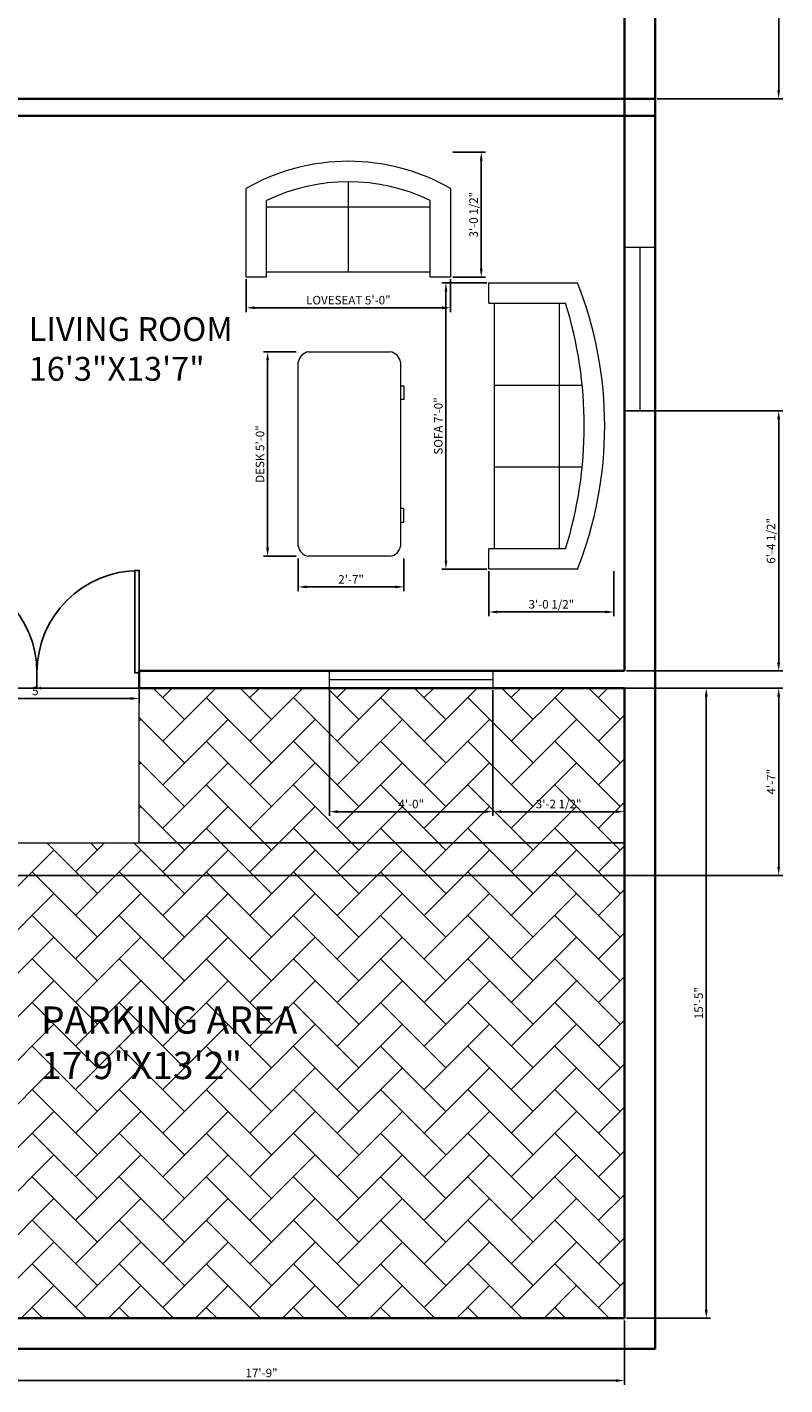
# Model space of a CAD drawing. Units: inches. Extents: x 3715 to 4224, y 2597 to 3354.
# Tile 3 of 5: x 4001 to 4224, y 2624 to 3023. Entities that reach past the tile are written whole.
import ezdxf

# ---------------------------------------------------------------- set-up
doc = ezdxf.new("R2010")
doc.units = ezdxf.units.IN
for name, color, linetype, lineweight in [('A-AREA-IDEN', 4, 'Continuous', 25), ('A-WALL', 7, 'Continuous', 35), ('DIM', 1, 'Continuous', 18), ('DOOR', 3, 'Continuous', 25), ('FURNITURES', 30, 'Continuous', 18), ('L-PAVE', 8, 'Continuous', 18), ('L-PAVE-PATT', 252, 'Continuous', 13), ('WINDOW', 6, 'Continuous', 20)]:
    doc.layers.add(name, color=color, linetype=linetype, lineweight=lineweight)
doc.styles.get("Standard").update_dxf_attribs({"font": 'arial.ttf'})
doc.dimstyles.new('ISO-25', dxfattribs={"dimtxt": 2.5, "dimasz": 2.5, "dimexe": 1.25, "dimexo": 0.625, "dimtad": 1, "dimlunit": 3, "dimtxsty": 'Standard', "dimcen": 2.5, "dimadec": 0, "dimazin": 0, "dimtfac": 1, "dimtmove": 0, "dimatfit": 3, "dimfxl": 1, "dimarcsym": 0})

# ---------------------------------------------------------------- blocks, each defined once
blk = doc.blocks.new('*U2')
for p, q in [((0, 0), (0, -6)), ((40, 0), (40, -6))]:
    blk.add_line(p, q)
blk.add_lwpolyline([(0, 0), (0, 40), (1.75, 40), (1.75, 0)], close=True)
blk.add_arc((0, 0), 40, 0, 90)
blk = doc.blocks.new('*U4')
for p, q in [((0, 0), (0, -6)), ((-40, 0), (-40, -6))]:
    blk.add_line(p, q)
blk.add_lwpolyline([(0, 0), (0, 40), (-1.75, 40), (-1.75, 0)], close=True)
blk.add_arc((0, 0), 40, 90, 180)
blk = doc.blocks.new('Desk - 30 x 60 in.')
for p, q in [((-26.999995, 0), (26.999995, 0)), ((-29.999995, -27), (-29.999995, -3)), ((29.999995, -3), (29.999995, -27)), ((26.999995, -30), (-26.999995, -30)), ((-20.000005, -30), (-20.000005, -31)), ((-20.000005, -31), (-16.000005, -31)), ((-16.000005, -31), (-16.000005, -30)), ((15.999995, -31), (15.999995, -30)), ((19.999995, -31), (15.999995, -31)), ((19.999995, -30), (19.999995, -31))]:
    blk.add_line(p, q)
for centre, start, end in [((-26.499995, -3.5), 98.1301, 171.8699), ((26.499995, -3.5), 8.130102, 81.8699), ((-26.499995, -26.5), 188.1301, 261.8699), ((26.499995, -26.5), 278.1301, 351.8699)]:
    blk.add_arc(centre, 3.535534, start, end)
blk = doc.blocks.new('Sofa - Roundback 7 ft.')
for p, q in [((-12.00002, -32.4421), (-12.00003, -6.5971)), ((11.99997, -32.4421), (11.99998, -6.5971)), ((-36.000027, -34), (-36.000027, -11.4696)), ((35.99998, -34), (35.99998, -11.4696)), ((-35.999844, -13.3819), (35.9998, -13.3819)), ((-36.000027, -32.4421), (35.99998, -32.4421))]:
    blk.add_line(p, q)
for points in [[(-36.000027, -34), (-42.000027, -34), (-42.000027, -8)], [(41.99998, -8), (41.99998, -34), (35.99998, -34)]]:
    blk.add_lwpolyline(points)
for centre, radius, start, end in [((0, -114.25), 114.25, 68.43141, 111.5686), ((-0.00001, -127.1968), 121.1968, 72.72033, 107.2797)]:
    blk.add_arc(centre, radius, start, end)
blk = doc.blocks.new('Sofa - Roundback Loveseat 5 ft.')
for p, q in [((0, -32.44198), (0, -5.99998)), ((-24, -33.99998), (-24, -11.46958)), ((24.00004, -33.99998), (24.00004, -11.46958)), ((-23.9998, -13.38178), (23.99986, -13.38178)), ((-24, -32.44198), (24.00004, -32.44198))]:
    blk.add_line(p, q)
for points in [[(-24, -33.99998), (-30, -33.99998), (-30, -7.99998)], [(30.00004, -7.99998), (30.00004, -33.99998), (24.00004, -33.99998)]]:
    blk.add_lwpolyline(points)
for centre, radius, start, end in [((0, -60.24998), 60.24998, 60.13715, 119.8628), ((0, -61.38438), 55.38444, 64.32083, 115.6792)]:
    blk.add_arc(centre, radius, start, end)
blk = doc.blocks.new('*D27')
at = {"layer": 'Defpoints', "color": 0, "transparency": 16777216}
for p in [(3963.48, 2643.93), (4176.48, 2643.93), (4176.48, 2625.63)]:
    blk.add_point(p, dxfattribs=at)
at = {"layer": 'DIM', "color": 0, "lineweight": -2, "transparency": 16777216}
for p, q in [((3963.48, 2643.31), (3963.48, 2624.38)), ((4176.48, 2643.31), (4176.48, 2624.38)), ((3965.98, 2625.63), (4173.98, 2625.63))]:
    blk.add_line(p, q, dxfattribs=at)
at = {"layer": 'DIM', "color": 0, "transparency": 16777216}
for points in [[(3965.98, 2626.04), (3965.98, 2625.21), (3963.48, 2625.63)], [(4173.98, 2626.04), (4173.98, 2625.21), (4176.48, 2625.63)]]:
    blk.add_solid(points, dxfattribs=at)
at = {"layer": 'DIM', "color": 0, "transparency": 16777216, "insert": (4069.98, 2627.53), "char_height": 2.5, "attachment_point": 5}
blk.add_mtext('17\'-9"', dxfattribs=at)
blk = doc.blocks.new('*D28')
at = {"layer": 'Defpoints', "color": 0, "transparency": 16777216}
for p in [(4176.48, 2828.93), (4176.48, 2643.93), (4200.53, 2643.93)]:
    blk.add_point(p, dxfattribs=at)
at = {"layer": 'DIM', "color": 0, "lineweight": -2, "transparency": 16777216}
for p, q in [((4177.1, 2828.93), (4201.78, 2828.93)), ((4200.53, 2826.43), (4200.53, 2646.43)), ((4177.1, 2643.93), (4201.78, 2643.93))]:
    blk.add_line(p, q, dxfattribs=at)
at = {"layer": 'DIM', "color": 0, "transparency": 16777216}
for points in [[(4200.11, 2826.43), (4200.95, 2826.43), (4200.53, 2828.93)], [(4200.11, 2646.43), (4200.95, 2646.43), (4200.53, 2643.93)]]:
    blk.add_solid(points, dxfattribs=at)
at = {"layer": 'DIM', "color": 0, "transparency": 16777216, "insert": (4198.63, 2736.43), "char_height": 2.5, "attachment_point": 5, "rotation": 90}
blk.add_mtext('15\'-5"', dxfattribs=at)
blk = doc.blocks.new('*D35')
at = {"layer": 'Defpoints', "color": 0, "transparency": 16777216}
for p in [(3974.06, 2828.93), (4034.06, 2828.93), (4034.06, 2825.86)]:
    blk.add_point(p, dxfattribs=at)
at = {"layer": 'DIM', "color": 0, "lineweight": -2, "transparency": 16777216}
for p, q in [((3974.06, 2828.31), (3974.06, 2824.61)), ((3976.56, 2825.86), (4031.56, 2825.86)), ((4034.06, 2828.31), (4034.06, 2824.61))]:
    blk.add_line(p, q, dxfattribs=at)
at = {"layer": 'DIM', "color": 0, "transparency": 16777216}
for points in [[(3976.56, 2826.28), (3976.56, 2825.45), (3974.06, 2825.86)], [(4031.56, 2826.28), (4031.56, 2825.45), (4034.06, 2825.86)]]:
    blk.add_solid(points, dxfattribs=at)
at = {"layer": 'DIM', "color": 0, "transparency": 16777216, "insert": (4004.06, 2827.76), "char_height": 2.5, "attachment_point": 5}
blk.add_mtext("5'", dxfattribs=at)
blk = doc.blocks.new('WIN-48IN-9IN-WALL')
blk.add_line((4.5, 48), (4.5, 0))
blk.add_lwpolyline([(0, 48), (9, 48), (9, 0), (0, 0)], close=True)
blk = doc.blocks.new('*D57')
at = {"layer": 'Defpoints', "color": 0, "transparency": 16777216}
for p in [(4071.76, 2927.61), (4080.76, 2927.61), (4080.76, 2867.61)]:
    blk.add_point(p, dxfattribs=at)
at = {"layer": 'DIM', "color": 0, "lineweight": -2, "transparency": 16777216}
for p, q in [((4080.14, 2927.61), (4070.51, 2927.61)), ((4071.76, 2870.11), (4071.76, 2925.11)), ((4080.14, 2867.61), (4070.51, 2867.61))]:
    blk.add_line(p, q, dxfattribs=at)
at = {"layer": 'DIM', "color": 0, "transparency": 16777216}
for points in [[(4071.35, 2925.11), (4072.18, 2925.11), (4071.76, 2927.61)], [(4071.35, 2870.11), (4072.18, 2870.11), (4071.76, 2867.61)]]:
    blk.add_solid(points, dxfattribs=at)
at = {"layer": 'DIM', "color": 0, "transparency": 16777216, "insert": (4069.85, 2897.61), "char_height": 2.5, "attachment_point": 5, "rotation": 90}
blk.add_mtext('DESK 5\'-0"', dxfattribs=at)
blk = doc.blocks.new('*D58')
at = {"layer": 'Defpoints', "color": 0, "transparency": 16777216}
for p in [(4080.76, 2867.61), (4111.76, 2867.61), (4080.76, 2858.61)]:
    blk.add_point(p, dxfattribs=at)
at = {"layer": 'DIM', "color": 0, "lineweight": -2, "transparency": 16777216}
for p, q in [((4080.76, 2866.98), (4080.76, 2857.36)), ((4111.76, 2866.98), (4111.76, 2857.36)), ((4109.26, 2858.61), (4083.26, 2858.61))]:
    blk.add_line(p, q, dxfattribs=at)
at = {"layer": 'DIM', "color": 0, "transparency": 16777216}
for points in [[(4083.26, 2859.02), (4083.26, 2858.19), (4080.76, 2858.61)], [(4109.26, 2859.02), (4109.26, 2858.19), (4111.76, 2858.61)]]:
    blk.add_solid(points, dxfattribs=at)
at = {"layer": 'DIM', "color": 0, "transparency": 16777216, "insert": (4096.26, 2860.49), "char_height": 2.5, "attachment_point": 5}
blk.add_mtext('2\'-7"', dxfattribs=at)
blk = doc.blocks.new('*D61')
at = {"layer": 'Defpoints', "color": 0, "transparency": 16777216}
for p in [(4136.71, 2947.86), (4124.11, 2863.86), (4136.71, 2863.86)]:
    blk.add_point(p, dxfattribs=at)
at = {"layer": 'DIM', "color": 0, "lineweight": -2, "transparency": 16777216}
for p, q in [((4136.09, 2947.86), (4122.86, 2947.86)), ((4124.11, 2945.36), (4124.11, 2866.36)), ((4136.09, 2863.86), (4122.86, 2863.86))]:
    blk.add_line(p, q, dxfattribs=at)
at = {"layer": 'DIM', "color": 0, "transparency": 16777216}
for points in [[(4123.7, 2945.36), (4124.53, 2945.36), (4124.11, 2947.86)], [(4123.7, 2866.36), (4124.53, 2866.36), (4124.11, 2863.86)]]:
    blk.add_solid(points, dxfattribs=at)
at = {"layer": 'DIM', "color": 0, "transparency": 16777216, "insert": (4122.19, 2905.86), "char_height": 2.5, "attachment_point": 5, "rotation": 90}
blk.add_mtext('SOFA 7\'-0"', dxfattribs=at)
blk = doc.blocks.new('*D62')
at = {"layer": 'Defpoints', "color": 0, "transparency": 16777216}
for p in [(4136.71, 2863.86), (4173.38, 2863.86), (4173.38, 2851.26)]:
    blk.add_point(p, dxfattribs=at)
at = {"layer": 'DIM', "color": 0, "lineweight": -2, "transparency": 16777216}
for p, q in [((4136.71, 2863.24), (4136.71, 2850.01)), ((4173.38, 2863.24), (4173.38, 2850.01)), ((4139.21, 2851.26), (4170.88, 2851.26))]:
    blk.add_line(p, q, dxfattribs=at)
at = {"layer": 'DIM', "color": 0, "transparency": 16777216}
for points in [[(4139.21, 2851.68), (4139.21, 2850.84), (4136.71, 2851.26)], [(4170.88, 2851.68), (4170.88, 2850.84), (4173.38, 2851.26)]]:
    blk.add_solid(points, dxfattribs=at)
at = {"layer": 'DIM', "color": 0, "transparency": 16777216, "insert": (4155.05, 2853.18), "char_height": 2.5, "attachment_point": 5}
blk.add_mtext('3\'-0 1/2"', dxfattribs=at)
blk = doc.blocks.new('*D63')
at = {"layer": 'Defpoints', "color": 0, "transparency": 16777216}
for p in [(4065.47, 2949.55), (4125.47, 2949.55), (4125.47, 2940.55)]:
    blk.add_point(p, dxfattribs=at)
at = {"layer": 'DIM', "color": 0, "lineweight": -2, "transparency": 16777216}
for p, q in [((4065.47, 2948.93), (4065.47, 2939.3)), ((4125.47, 2948.93), (4125.47, 2939.3)), ((4067.97, 2940.55), (4122.97, 2940.55))]:
    blk.add_line(p, q, dxfattribs=at)
at = {"layer": 'DIM', "color": 0, "transparency": 16777216}
for points in [[(4067.97, 2940.97), (4067.97, 2940.14), (4065.47, 2940.55)], [(4122.97, 2940.97), (4122.97, 2940.14), (4125.47, 2940.55)]]:
    blk.add_solid(points, dxfattribs=at)
at = {"layer": 'DIM', "color": 0, "transparency": 16777216, "insert": (4095.47, 2942.47), "char_height": 2.5, "attachment_point": 5}
blk.add_mtext('LOVESEAT 5\'-0"', dxfattribs=at)
blk = doc.blocks.new('*D64')
at = {"layer": 'Defpoints', "color": 0, "transparency": 16777216}
for p in [(4125.47, 2986.22), (4134.47, 2986.22), (4125.47, 2949.55)]:
    blk.add_point(p, dxfattribs=at)
at = {"layer": 'DIM', "color": 0, "lineweight": -2, "transparency": 16777216}
for p, q in [((4126.09, 2986.22), (4135.72, 2986.22)), ((4134.47, 2952.05), (4134.47, 2983.72)), ((4126.09, 2949.55), (4135.72, 2949.55))]:
    blk.add_line(p, q, dxfattribs=at)
at = {"layer": 'DIM', "color": 0, "transparency": 16777216}
for points in [[(4134.05, 2983.72), (4134.88, 2983.72), (4134.47, 2986.22)], [(4134.05, 2952.05), (4134.88, 2952.05), (4134.47, 2949.55)]]:
    blk.add_solid(points, dxfattribs=at)
at = {"layer": 'DIM', "color": 0, "transparency": 16777216, "insert": (4132.55, 2967.89), "char_height": 2.5, "attachment_point": 5, "rotation": 90}
blk.add_mtext('3\'-0 1/2"', dxfattribs=at)
blk = doc.blocks.new('*D82')
at = {"layer": 'Defpoints', "color": 0, "transparency": 16777216}
for p in [(3958.48, 2828.93), (4221.78, 2828.93), (3963.48, 2773.93)]:
    blk.add_point(p, dxfattribs=at)
at = {"layer": 'DIM', "color": 0, "lineweight": -2, "transparency": 16777216}
for p, q in [((3959.1, 2828.93), (4223.03, 2828.93)), ((4221.78, 2776.43), (4221.78, 2826.43)), ((3964.1, 2773.93), (4223.03, 2773.93))]:
    blk.add_line(p, q, dxfattribs=at)
at = {"layer": 'DIM', "color": 0, "transparency": 16777216}
for points in [[(4221.36, 2826.43), (4222.19, 2826.43), (4221.78, 2828.93)], [(4221.36, 2776.43), (4222.19, 2776.43), (4221.78, 2773.93)]]:
    blk.add_solid(points, dxfattribs=at)
at = {"layer": 'DIM', "color": 0, "transparency": 16777216, "insert": (4219.9, 2801.43), "char_height": 2.5, "attachment_point": 5, "rotation": 90}
blk.add_mtext('4\'-7"', dxfattribs=at)
blk = doc.blocks.new('*D86')
at = {"layer": 'Defpoints', "color": 0, "transparency": 16777216}
for p in [(4176.48, 2910.33), (4221.78, 2910.33), (4176.48, 2833.93)]:
    blk.add_point(p, dxfattribs=at)
at = {"layer": 'DIM', "color": 0, "lineweight": -2, "transparency": 16777216}
for p, q in [((4177.1, 2910.33), (4223.03, 2910.33)), ((4221.78, 2836.43), (4221.78, 2907.83)), ((4177.1, 2833.93), (4223.03, 2833.93))]:
    blk.add_line(p, q, dxfattribs=at)
at = {"layer": 'DIM', "color": 0, "transparency": 16777216}
for points in [[(4221.36, 2907.83), (4222.19, 2907.83), (4221.78, 2910.33)], [(4221.36, 2836.43), (4222.19, 2836.43), (4221.78, 2833.93)]]:
    blk.add_solid(points, dxfattribs=at)
at = {"layer": 'DIM', "color": 0, "transparency": 16777216, "insert": (4219.86, 2872.13), "char_height": 2.5, "attachment_point": 5, "rotation": 90}
blk.add_mtext('6\'-4 1/2"', dxfattribs=at)
blk = doc.blocks.new('*D87')
at = {"layer": 'Defpoints', "color": 0, "transparency": 16777216}
for p in [(4176.48, 3062.95), (4221.78, 3062.95), (4185.48, 3001.93)]:
    blk.add_point(p, dxfattribs=at)
at = {"layer": 'DIM', "color": 0, "lineweight": -2, "transparency": 16777216}
for p, q in [((4177.1, 3062.95), (4223.03, 3062.95)), ((4221.78, 3004.43), (4221.78, 3060.45)), ((4186.1, 3001.93), (4223.03, 3001.93))]:
    blk.add_line(p, q, dxfattribs=at)
at = {"layer": 'DIM', "color": 0, "transparency": 16777216}
for points in [[(4221.36, 3060.45), (4222.19, 3060.45), (4221.78, 3062.95)], [(4221.36, 3004.43), (4222.19, 3004.43), (4221.78, 3001.93)]]:
    blk.add_solid(points, dxfattribs=at)
at = {"layer": 'DIM', "color": 0, "transparency": 16777216, "insert": (4219.87, 3032.44), "char_height": 2.5, "attachment_point": 5, "rotation": 90}
blk.add_mtext('5\'-1"', dxfattribs=at)
blk = doc.blocks.new('*D93')
at = {"layer": 'Defpoints', "color": 0, "transparency": 16777216}
for p in [(4089.91, 2828.93), (4137.91, 2828.93), (4089.91, 2792.63)]:
    blk.add_point(p, dxfattribs=at)
at = {"layer": 'DIM', "color": 0, "lineweight": -2, "transparency": 16777216}
for p, q in [((4089.91, 2828.31), (4089.91, 2791.38)), ((4137.91, 2828.31), (4137.91, 2791.38)), ((4135.41, 2792.63), (4092.41, 2792.63))]:
    blk.add_line(p, q, dxfattribs=at)
at = {"layer": 'DIM', "color": 0, "transparency": 16777216}
for points in [[(4092.41, 2793.05), (4092.41, 2792.22), (4089.91, 2792.63)], [(4135.41, 2793.05), (4135.41, 2792.22), (4137.91, 2792.63)]]:
    blk.add_solid(points, dxfattribs=at)
at = {"layer": 'DIM', "color": 0, "transparency": 16777216, "insert": (4113.91, 2794.54), "char_height": 2.5, "attachment_point": 5}
blk.add_mtext('4\'-0"', dxfattribs=at)
blk = doc.blocks.new('*D94')
at = {"layer": 'Defpoints', "color": 0, "transparency": 16777216}
for p in [(4137.91, 2828.93), (4176.48, 2828.93), (4137.91, 2792.63)]:
    blk.add_point(p, dxfattribs=at)
at = {"layer": 'DIM', "color": 0, "lineweight": -2, "transparency": 16777216}
for p, q in [((4137.91, 2828.31), (4137.91, 2791.38)), ((4176.48, 2828.31), (4176.48, 2791.38)), ((4173.98, 2792.63), (4140.41, 2792.63))]:
    blk.add_line(p, q, dxfattribs=at)
at = {"layer": 'DIM', "color": 0, "transparency": 16777216}
for points in [[(4140.41, 2793.05), (4140.41, 2792.22), (4137.91, 2792.63)], [(4173.98, 2793.05), (4173.98, 2792.22), (4176.48, 2792.63)]]:
    blk.add_solid(points, dxfattribs=at)
at = {"layer": 'DIM', "color": 0, "transparency": 16777216, "insert": (4157.19, 2794.55), "char_height": 2.5, "attachment_point": 5}
blk.add_mtext('3\'-2 1/2"', dxfattribs=at)

msp = doc.modelspace()

# ---------------------------------------------------------------- hatches: boundary and pattern name
at = {"layer": 'L-PAVE-PATT', "transparency": 33554508}
h = msp.add_hatch(dxfattribs=at)
h.set_pattern_fill('AR-HBONE', color=256, scale=0.089)
h.paths.add_polyline_path([(4176.476, 2783.444), (4034.058, 2783.444), (3963.476, 2783.444), (3963.476, 2643.934), (4176.476, 2643.934)])
h.paths.add_polyline_path([(4176.476, 2828.934), (4034.058, 2828.934), (4034.058, 2783.444), (4176.476, 2783.444)])

# ---------------------------------------------------------------- linework, layer by layer
at = {"layer": 'A-WALL'}
for p, q in [((4185.476, 2634.934), (4185.476, 3311.934)), ((4176.476, 2833.934), (4176.476, 3164.934)), ((3963.476, 3001.934), (4185.476, 3001.934)), ((3963.476, 2996.934), (4185.476, 2996.934)), ((4034.058, 2833.934), (4176.476, 2833.934)), ((4034.058, 2828.934), (4176.476, 2828.934)), ((4176.476, 2643.934), (4176.476, 2828.934)), ((3765.476, 2643.934), (4176.476, 2643.934)), ((3756.476, 2634.934), (4185.476, 2634.934))]:
    msp.add_line(p, q, dxfattribs=at)
msp.add_lwpolyline([(4034.058, 2833.934), (4034.058, 2828.934)], dxfattribs=at)
at = {"layer": 'L-PAVE'}
for points in [[(4034.058, 2828.934), (4176.476, 2828.934), (4176.476, 2783.444), (4034.058, 2783.444)], [(3963.476, 2783.444), (4176.476, 2783.444), (4176.476, 2643.934), (3963.476, 2643.934)]]:
    msp.add_lwpolyline(points, close=True, dxfattribs=at)
at = {"layer": 'WINDOW'}
msp.add_line((4089.914, 2831.434), (4137.914, 2831.434), dxfattribs=at)
msp.add_lwpolyline([(4089.914, 2828.934), (4089.914, 2833.934), (4137.914, 2833.934), (4137.914, 2828.934)], close=True, dxfattribs=at)

# ---------------------------------------------------------------- block references
at = {"layer": 'DOOR', "xscale": 0.75, "yscale": 0.75, "zscale": 0.75}
for name, p in [('*U2', (3974.058, 2833.434)), ('*U4', (4034.058, 2833.434))]:
    msp.add_blockref(name, p, dxfattribs=at)
at = {"layer": 'FURNITURES'}
msp.add_blockref('Sofa - Roundback Loveseat 5 ft.', (4095.466, 2983.552), dxfattribs=at)
for name, p, rotation in [('Sofa - Roundback 7 ft.', (4170.712, 2905.861), 270), ('Desk - 30 x 60 in.', (4080.764, 2897.606), 90)]:
    msp.add_blockref(name, p, dxfattribs=dict(at, rotation=rotation))
at = {"layer": 'WINDOW'}
msp.add_blockref('WIN-48IN-9IN-WALL', (4176.476, 2910.33), dxfattribs=at)

# ---------------------------------------------------------------- texts
at = {"layer": 'A-AREA-IDEN', "attachment_point": 1}
for s, insert, char_height in [('LIVING ROOM\\P16\'3"X13\'7"', (4001.642, 2937.801), 7), ('PARKING AREA\\P17\'9"X13\'2"', (4005.261, 2735.458), 8)]:
    msp.add_mtext_dynamic_manual_height_columns(s, width=94.29963, gutter_width=12.5, heights=[0], dxfattribs=dict(at, insert=insert, char_height=char_height))

# ---------------------------------------------------------------- dimensions: what is measured, and where the dimension line sits
at = {"layer": 'DIM'}
for base, p1, p2, angle, override, picture, middle in [((4221.776, 3062.946), (4185.476, 3001.934), (4176.476, 3062.946), 90, {"dimdec": 1, "dimlfac": 1, "dimrnd": 0, "dimzin": 1, "dimdsep": 46, "dimlunit": 4, "dimfrac": 2}, '*D87', (4219.874, 3032.44)), ((4134.466, 2986.219), (4125.466, 2949.552), (4125.466, 2986.219), 90, {"dimdec": 1, "dimlfac": 1, "dimrnd": 0, "dimzin": 1, "dimdsep": 46, "dimlunit": 4, "dimfrac": 2}, '*D64', (4132.547, 2967.885)), ((4221.776, 2910.329), (4176.476, 2833.934), (4176.476, 2910.329), 90, {"dimdec": 1, "dimlfac": 1, "dimrnd": 0, "dimzin": 1, "dimdsep": 46, "dimlunit": 4, "dimfrac": 2}, '*D86', (4219.858, 2872.132)), ((4080.764, 2858.606), (4111.764, 2867.606), (4080.764, 2867.606), 180, {"dimdec": 1, "dimlfac": 1, "dimrnd": 0, "dimzin": 1, "dimdsep": 46, "dimlunit": 4, "dimfrac": 2}, '*D58', (4096.264, 2860.487)), ((4221.776, 2828.934), (3963.476, 2773.934), (3958.476, 2828.934), 90, {"dimdec": 1, "dimlfac": 1, "dimrnd": 0, "dimzin": 1, "dimdsep": 46, "dimlunit": 4, "dimfrac": 2}, '*D82', (4219.901, 2801.434)), ((4089.914, 2792.634), (4137.914, 2828.934), (4089.914, 2828.934), 180, {"dimdec": 1, "dimlfac": 1, "dimrnd": 0, "dimzin": 1, "dimdsep": 46, "dimlunit": 4, "dimfrac": 2}, '*D93', (4113.914, 2794.535)), ((4137.914, 2792.634), (4176.476, 2828.934), (4137.914, 2828.934), 180, {"dimdec": 1, "dimlfac": 1, "dimrnd": 0, "dimzin": 1, "dimdsep": 46, "dimlunit": 4, "dimfrac": 2}, '*D94', (4157.195, 2794.552)), ((4200.531, 2643.934), (4176.476, 2828.934), (4176.476, 2643.934), 90, {"dimclrd": 0, "dimclre": 0, "dimclrt": 0}, '*D28', (4198.629, 2736.434))]:
    dim = msp.add_linear_dim(base=base, p1=p1, p2=p2, angle=angle, dimstyle='ISO-25', override=override, dxfattribs=at)
    dim.commit()
    dim.dimension.update_dxf_attribs({"geometry": picture, "text_midpoint": middle})
dim = msp.add_linear_dim(base=(4125.466, 2940.552), p1=(4065.466, 2949.552), p2=(4125.466, 2949.552), text='LOVESEAT <>', dimstyle='ISO-25', override={"dimdec": 1, "dimlfac": 1, "dimrnd": 0, "dimzin": 1, "dimdsep": 46, "dimlunit": 4, "dimfrac": 2}, dxfattribs=at)
dim.commit()
dim.dimension.update_dxf_attribs({"geometry": '*D63', "text_midpoint": (4095.466, 2942.47)})
for base, p1, p2, angle, text, picture, middle in [((4124.112, 2863.861), (4136.712, 2947.861), (4136.712, 2863.861), 270, 'SOFA <>', '*D61', (4122.194, 2905.861)), ((4071.764, 2927.606), (4080.764, 2867.606), (4080.764, 2927.606), 90, 'DESK <>', '*D57', (4069.846, 2897.606))]:
    dim = msp.add_linear_dim(base=base, p1=p1, p2=p2, angle=angle, text=text, dimstyle='ISO-25', override={"dimdec": 1, "dimlfac": 1, "dimrnd": 0, "dimzin": 1, "dimdsep": 46, "dimlunit": 4, "dimfrac": 2}, dxfattribs=at)
    dim.commit()
    dim.dimension.update_dxf_attribs({"geometry": picture, "text_midpoint": middle})
for base, p1, p2, override, picture, middle in [((4173.379, 2851.261), (4136.712, 2863.861), (4173.379, 2863.861), {"dimdec": 1, "dimlfac": 1, "dimrnd": 0, "dimzin": 1, "dimdsep": 46, "dimlunit": 4, "dimfrac": 2}, '*D62', (4155.046, 2853.179)), ((4034.058, 2825.862), (3974.058, 2828.934), (4034.058, 2828.934), {"dimclrd": 0, "dimclre": 0, "dimclrt": 0}, '*D35', (4004.058, 2827.758)), ((4176.476, 2625.625), (3963.476, 2643.934), (4176.476, 2643.934), {"dimclrd": 0, "dimclre": 0, "dimclrt": 0}, '*D27', (4069.976, 2627.527))]:
    dim = msp.add_linear_dim(base=base, p1=p1, p2=p2, dimstyle='ISO-25', override=override, dxfattribs=at)
    dim.commit()
    dim.dimension.update_dxf_attribs({"geometry": picture, "text_midpoint": middle})

doc.saveas('drawing.dxf')
